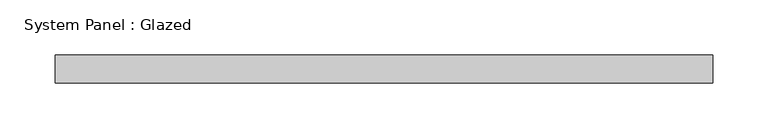
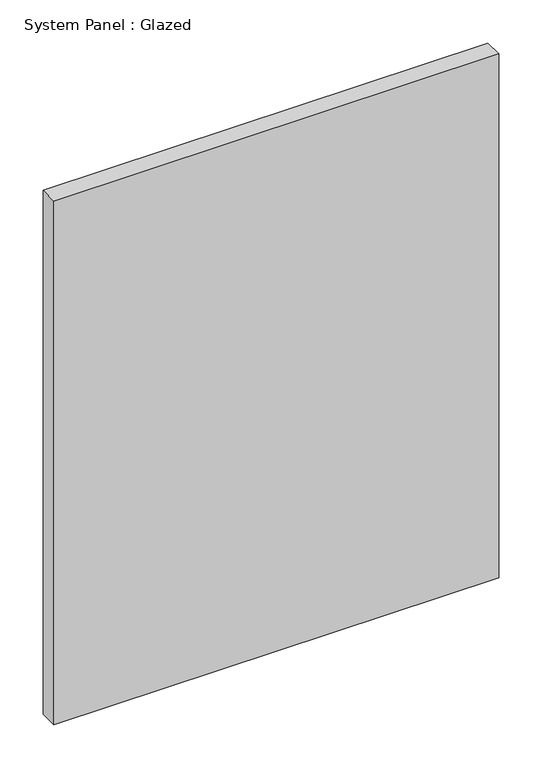
"""IFC4 building model written with IfcOpenShell, lengths in millimetres: plate geometry, System Panel : Glazed."""

from ifc_helpers import new_model, si_unit, origin, origin_with_axes, place, context, project, spatial, polyline, outline, extrude, source, transform, mapped, element, save


def system_panel_glazed_06a12247(model_context):
    return source(origin(), model_context, "Body", "SweptSolid", [
        extrude(outline(polyline([(298.45, 19.05), (-298.45, 19.05), (-298.45, 44.45), (298.45, 44.45), (298.45, 19.05)])), origin_with_axes(), (0.0, 0.0, 1.0), 742.95),
    ])


if __name__ == "__main__":
    model = new_model("IFC4")
    model_context = context("Model", 3, world=origin())
    ifc_project = project(units=[si_unit("LENGTHUNIT", "METRE", prefix="MILLI")], contexts=[model_context])
    site = spatial("IfcSite", under=ifc_project)
    building = spatial("IfcBuilding", under=site)
    placement = place(None, origin())
    system_panel_glazed_shape = system_panel_glazed_06a12247(model_context)
    element("IfcPlate", 1, ObjectType="System Panel : Glazed", at=placement, inside=building, context=model_context, shape_type="MappedRepresentation", body=[
        mapped(system_panel_glazed_shape, transform((0.0, 0.0, 0.0), x_axis=(1.0, 0.0, 0.0), y_axis=(0.0, 1.0, 0.0), z_axis=(0.0, 0.0, 1.0))),
    ])
    save(model, "model.ifc")

# Revit data of these elements
# Type "System Panel : Glazed"
#   Construction Type Id = "GSP4R"
#   Analytic Construction = "1/8 in Pilkington single glazing"
#   Visual Light Transmittance = 0.9
#   Solar Heat Gain Coefficient = 0.86
#   Heat Transfer Coefficient (U) = 1.18115 BTU/(h·ft²·°F)
#   Define Thermal Properties by = 1
# Element 1 (IfcPlate, "System Panel : Glazed")
#   Materials on its faces: "Glass"
# Materials
#   "Glass": class "Glass", colour RGB 0 128 192, transparency 0.75, Description = "Soda Lime Glass", Cost = 0
